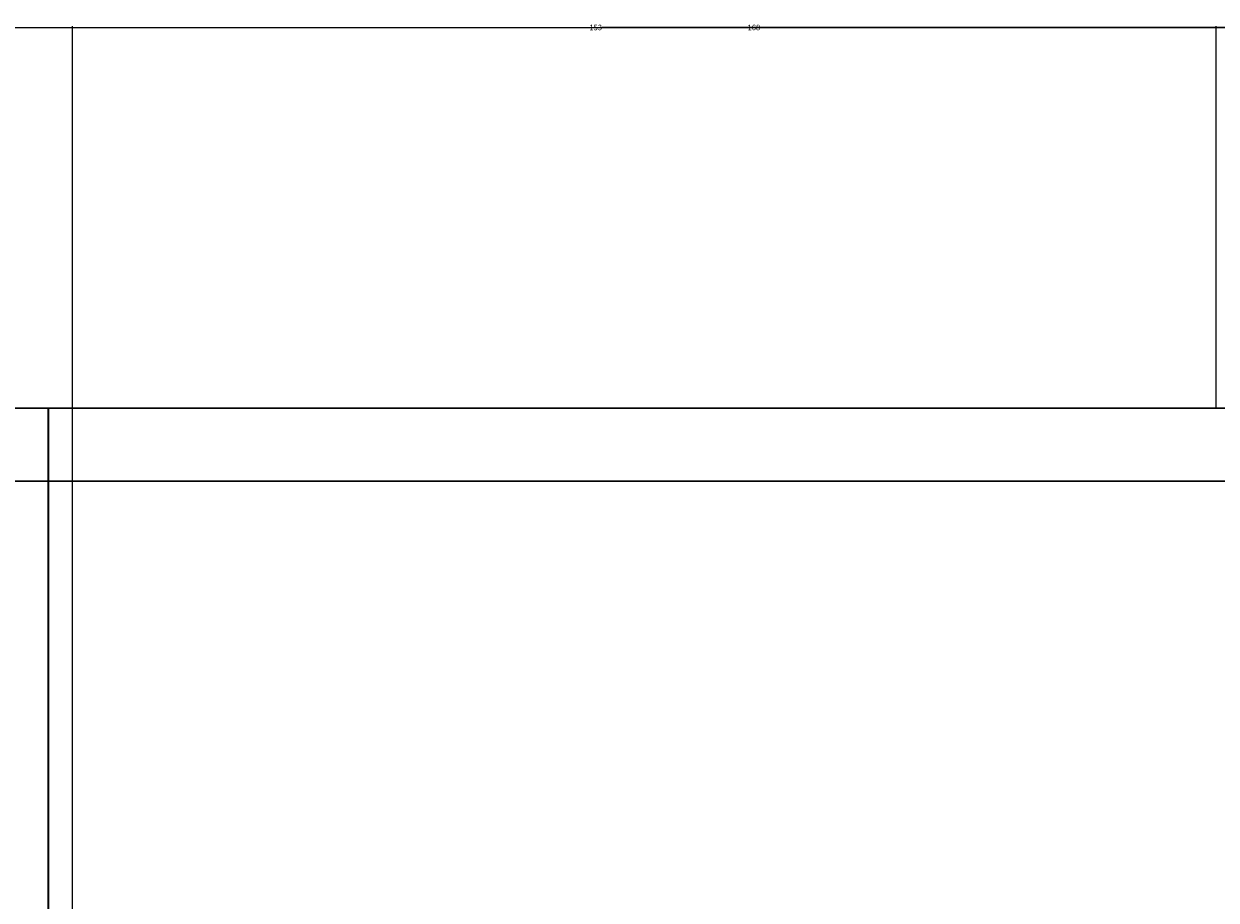
# Model space of a CAD drawing. Units: inches. Extents: x 867 to 1667, y -234 to 788.
# Tile 33 of 42: x 1074 to 1221, y 680 to 788. Entities that reach past the tile are written whole.
import ezdxf

# ---------------------------------------------------------------- set-up
doc = ezdxf.new("R2010")
doc.units = ezdxf.units.IN
doc.header["$MEASUREMENT"] = 0
for name, color, linetype, lineweight in [('A-ANNO-DIMS', 2, 'Continuous', 18), ('A-Wall', 7, 'Continuous', 35), ('A-WALL-SITE', 8, 'Continuous', 30)]:
    doc.layers.add(name, color=color, linetype=linetype, lineweight=lineweight)
doc.styles.get("Standard").update_dxf_attribs({"font": 'arial.ttf'})
doc.dimstyles.get("Standard").update_dxf_attribs({"dimtxt": 0.6875, "dimasz": 0.18, "dimexe": 0.18, "dimexo": 0.0625, "dimgap": 0.09, "dimtad": 0, "dimdec": 4, "dimzin": 0, "dimdsep": 46, "dimlunit": 4, "dimtxsty": 'Standard', "dimcen": 0.09, "dimadec": 0, "dimazin": 0, "dimtfac": 1, "dimtdec": 4, "dimtofl": 0, "dimtmove": 0, "dimatfit": 3, "dimfxl": 1, "dimtolj": 1, "dimtzin": 0, "dimarcsym": 0})

# ---------------------------------------------------------------- blocks, each defined once
blk = doc.blocks.new('*D17')
at = {"layer": 'A-ANNO-DIMS', "color": 0, "lineweight": -2, "transparency": 16777216}
for p, q in [((914.89, 740.68), (914.89, 787.75)), ((915.07, 787.57), (1266.54, 787.57)), ((1619.71, 787.57), (1268.24, 787.57)), ((1619.89, 740.68), (1619.89, 787.75))]:
    blk.add_line(p, q, dxfattribs=at)
at = {"layer": 'A-ANNO-DIMS', "color": 0, "transparency": 16777216}
for points in [[(915.07, 787.6), (915.07, 787.54), (914.89, 787.57)], [(1619.71, 787.6), (1619.71, 787.54), (1619.89, 787.57)]]:
    blk.add_solid(points, dxfattribs=at)
at = {"layer": 'Defpoints', "color": 0, "transparency": 16777216}
for p in [(1619.89, 787.57), (914.89, 740.62), (1619.89, 740.62)]:
    blk.add_point(p, dxfattribs=at)
at = {"layer": 'A-ANNO-DIMS', "color": 0, "transparency": 16777216, "insert": (1267.39, 787.57), "char_height": 0.688, "attachment_point": 5}
blk.add_mtext('\\A1;705', dxfattribs=at)
blk = doc.blocks.new('*D21')
at = {"layer": 'A-ANNO-DIMS', "color": 0, "lineweight": -2, "transparency": 16777216}
for p, q in [((1067.89, 740.68), (1067.89, 787.75)), ((1068.07, 787.57), (1143.57, 787.57)), ((1220.71, 787.57), (1145.2, 787.57)), ((1220.89, 740.68), (1220.89, 787.75))]:
    blk.add_line(p, q, dxfattribs=at)
at = {"layer": 'A-ANNO-DIMS', "color": 0, "transparency": 16777216}
for points in [[(1068.07, 787.6), (1068.07, 787.54), (1067.89, 787.57)], [(1220.71, 787.6), (1220.71, 787.54), (1220.89, 787.57)]]:
    blk.add_solid(points, dxfattribs=at)
at = {"layer": 'Defpoints', "color": 0, "transparency": 16777216}
for p in [(1220.89, 787.57), (1067.89, 740.62), (1220.89, 740.62)]:
    blk.add_point(p, dxfattribs=at)
at = {"layer": 'A-ANNO-DIMS', "color": 0, "transparency": 16777216, "insert": (1144.39, 787.57), "char_height": 0.688, "attachment_point": 5}
blk.add_mtext('\\A1;153', dxfattribs=at)
blk = doc.blocks.new('*D22')
at = {"layer": 'A-ANNO-DIMS', "color": 0, "lineweight": -2, "transparency": 16777216}
for p, q in [((1220.89, 740.68), (1220.89, 787.75)), ((1221.07, 787.57), (1301.07, 787.57)), ((1382.71, 787.57), (1302.7, 787.57)), ((1382.89, 740.68), (1382.89, 787.75))]:
    blk.add_line(p, q, dxfattribs=at)
at = {"layer": 'A-ANNO-DIMS', "color": 0, "transparency": 16777216}
for points in [[(1221.07, 787.6), (1221.07, 787.54), (1220.89, 787.57)], [(1382.71, 787.6), (1382.71, 787.54), (1382.89, 787.57)]]:
    blk.add_solid(points, dxfattribs=at)
at = {"layer": 'Defpoints', "color": 0, "transparency": 16777216}
for p in [(1382.89, 787.57), (1220.89, 740.62), (1382.89, 740.62)]:
    blk.add_point(p, dxfattribs=at)
at = {"layer": 'A-ANNO-DIMS', "color": 0, "transparency": 16777216, "insert": (1301.89, 787.57), "char_height": 0.688, "attachment_point": 5}
blk.add_mtext('\\A1;162', dxfattribs=at)
blk = doc.blocks.new('*D31')
at = {"layer": 'A-ANNO-DIMS', "color": 0, "lineweight": -2, "transparency": 16777216}
for p, q in [((1070.89, 566.68), (1070.89, 787.75)), ((1071.07, 787.57), (1304.02, 787.57)), ((1538.71, 787.57), (1305.75, 787.57)), ((1538.89, 566.68), (1538.89, 787.75))]:
    blk.add_line(p, q, dxfattribs=at)
at = {"layer": 'A-ANNO-DIMS', "color": 0, "transparency": 16777216}
for points in [[(1071.07, 787.6), (1071.07, 787.54), (1070.89, 787.57)], [(1538.71, 787.6), (1538.71, 787.54), (1538.89, 787.57)]]:
    blk.add_solid(points, dxfattribs=at)
at = {"layer": 'Defpoints', "color": 0, "transparency": 16777216}
for p in [(1538.89, 787.57), (1070.89, 566.62), (1538.89, 566.62)]:
    blk.add_point(p, dxfattribs=at)
at = {"layer": 'A-ANNO-DIMS', "color": 0, "transparency": 16777216, "insert": (1304.89, 787.57), "char_height": 0.688, "attachment_point": 5}
blk.add_mtext('\\A1;468', dxfattribs=at)
blk = doc.blocks.new('*D32')
at = {"layer": 'A-ANNO-DIMS', "color": 0, "lineweight": -2, "transparency": 16777216}
for p, q in [((1079.89, 404.68), (1079.89, 787.75)), ((1080.07, 787.57), (1163.07, 787.57)), ((1247.71, 787.57), (1164.7, 787.57)), ((1247.89, 413.68), (1247.89, 787.75))]:
    blk.add_line(p, q, dxfattribs=at)
at = {"layer": 'A-ANNO-DIMS', "color": 0, "transparency": 16777216}
for points in [[(1080.07, 787.6), (1080.07, 787.54), (1079.89, 787.57)], [(1247.71, 787.6), (1247.71, 787.54), (1247.89, 787.57)]]:
    blk.add_solid(points, dxfattribs=at)
at = {"layer": 'Defpoints', "color": 0, "transparency": 16777216}
for p in [(1247.89, 787.57), (1247.89, 413.62), (1079.89, 404.62)]:
    blk.add_point(p, dxfattribs=at)
at = {"layer": 'A-ANNO-DIMS', "color": 0, "transparency": 16777216, "insert": (1163.89, 787.57), "char_height": 0.688, "attachment_point": 5}
blk.add_mtext('\\A1;168', dxfattribs=at)

msp = doc.modelspace()

# ---------------------------------------------------------------- linework, layer by layer
at = {"layer": 'A-Wall'}
msp.add_line((1076.8866, 740.617), (1076.8866, 623.617), dxfattribs=at)
at = {"layer": 'A-WALL-SITE'}
for p, q in [((1619.8866, 740.617), (914.8866, 740.617)), ((1619.8866, 731.617), (914.8866, 731.617))]:
    msp.add_line(p, q, dxfattribs=at)

# ---------------------------------------------------------------- dimensions: what is measured, and where the dimension line sits
at = {"layer": 'A-ANNO-DIMS'}
for base, p1, p2, picture, middle in [((1619.8866, 787.567), (914.8866, 740.617), (1619.8866, 740.617), '*D17', (1267.3866, 787.567)), ((1220.8866, 787.567), (1067.8866, 740.617), (1220.8866, 740.617), '*D21', (1144.3866, 787.567)), ((1538.8866, 787.567), (1070.8866, 566.617), (1538.8866, 566.617), '*D31', (1304.8866, 787.567)), ((1247.8866, 787.567), (1079.8866, 404.617), (1247.8866, 413.617), '*D32', (1163.8866, 787.567)), ((1382.8866, 787.567), (1220.8866, 740.617), (1382.8866, 740.617), '*D22', (1301.8866, 787.567))]:
    dim = msp.add_linear_dim(base=base, p1=p1, p2=p2, dimstyle='Standard', override={"dimdec": 0, "dimlfac": 1, "dimrnd": 0, "dimzin": 0, "dimdsep": 46, "dimlunit": 2}, dxfattribs=at)
    dim.commit()
    dim.dimension.update_dxf_attribs({"geometry": picture, "text_midpoint": middle})

doc.saveas('drawing.dxf')
